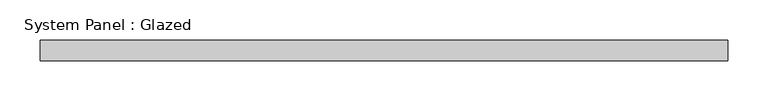
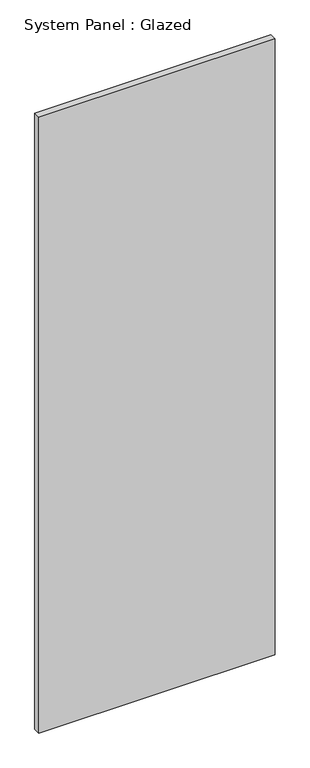
"""IFC4 building model written with IfcOpenShell, lengths in millimetres: plate geometry, System Panel : Glazed."""

from ifc_helpers import new_model, si_unit, origin, origin_with_axes, place, context, project, spatial, polyline, outline, extrude, source, transform, mapped, element, save


def system_panel_glazed_2937bf4c(model_context):
    return source(origin(), model_context, "Body", "SweptSolid", [
        extrude(outline(polyline([(425.45, -44.45), (-425.45, -44.45), (-425.45, -19.05), (425.45, -19.05), (425.45, -44.45)])), origin_with_axes(), (0.0, 0.0, 1.0), 2343.15),
    ])


if __name__ == "__main__":
    model = new_model("IFC4")
    model_context = context("Model", 3, world=origin())
    ifc_project = project(units=[si_unit("LENGTHUNIT", "METRE", prefix="MILLI")], contexts=[model_context])
    site = spatial("IfcSite", under=ifc_project)
    building = spatial("IfcBuilding", under=site)
    placement = place(None, origin())
    system_panel_glazed_shape = system_panel_glazed_2937bf4c(model_context)
    element("IfcPlate", 1, ObjectType="System Panel : Glazed", at=placement, inside=building, context=model_context, shape_type="MappedRepresentation", body=[
        mapped(system_panel_glazed_shape, transform((0.0, 0.0, 0.0), x_axis=(1.0, 0.0, 0.0), y_axis=(0.0, 1.0, 0.0), z_axis=(0.0, 0.0, 1.0))),
    ])
    save(model, "model.ifc")

# Revit data of these elements
# Type "System Panel : Glazed"
#   Construction Type Id = "GSP4R"
#   Analytic Construction = "1/8 in Pilkington single glazing"
#   Visual Light Transmittance = 0.9
#   Solar Heat Gain Coefficient = 0.86
#   Heat Transfer Coefficient (U) = 1.18115 BTU/(h·ft²·°F)
# Element 1 (IfcPlate, "System Panel : Glazed")
#   Materials on its faces: "Glass"
# Materials
#   "Glass": class "Glass", colour RGB 0 128 192, transparency 0.75, Description = "Soda Lime Glass", Cost = 0
